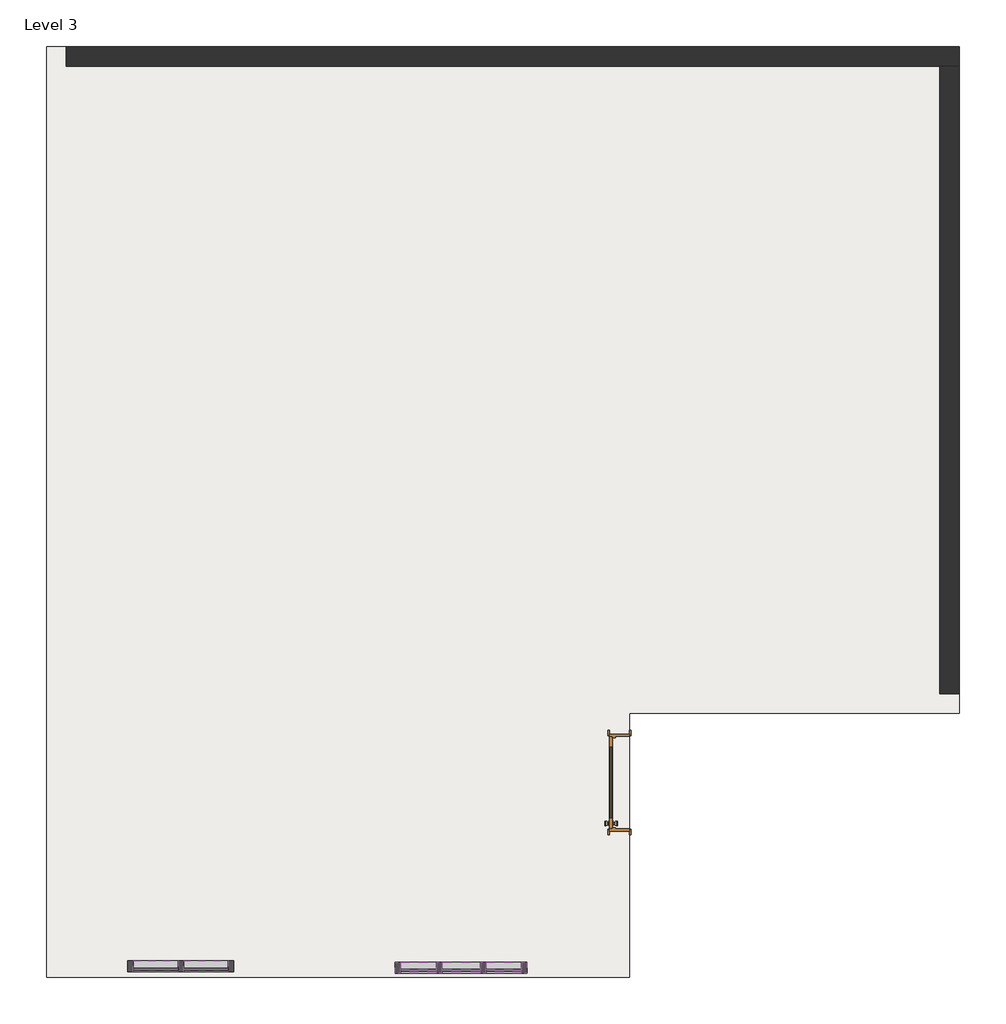
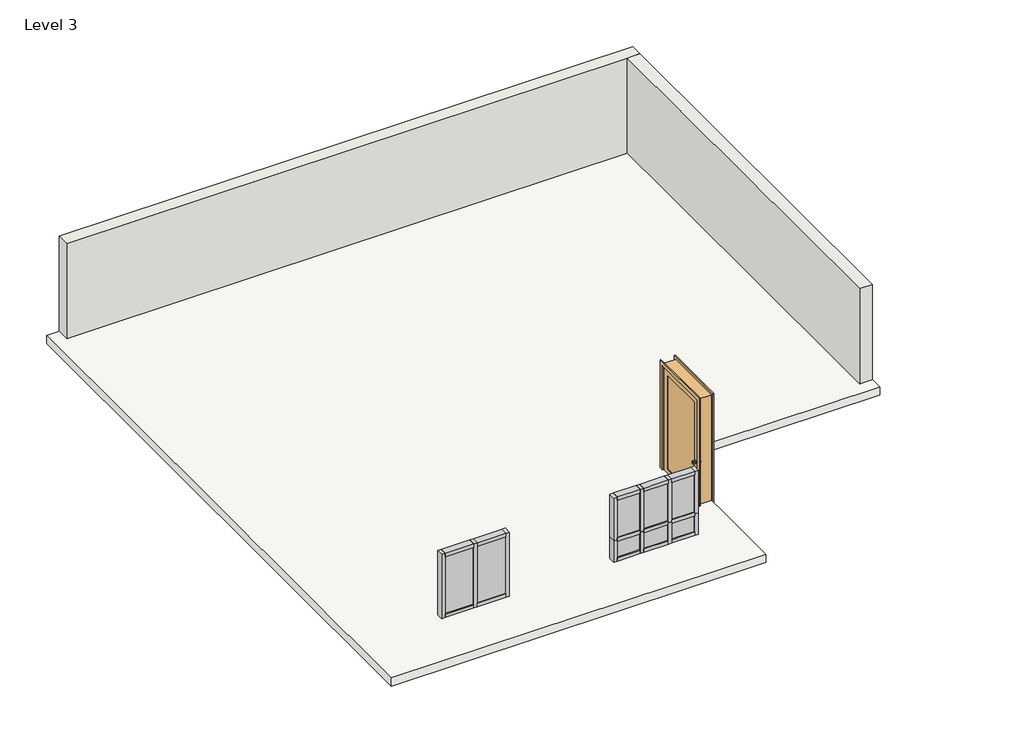
# One storey: 24 members, 8 plates, 2 walls, 1 door, 1 roof.
"""IFC4 building model written with IfcOpenShell, lengths in millimetres."""

from ifc_helpers import new_model, si_unit, frame, origin, place, context, project, spatial, polyline, outline, extrude, faceted_brep, transform, mapped, element, save
from components import door_103cf79b, member_0b7646a3, member_2b49869a, member_75074519, member_dc106669, member_90c805a2, member_5ae8a700, member_718fe5d9, member_bc7dbe04, member_58a4a87b, member_8b3492ed, member_7cfea1b5, system_panel_glazed_1715a493, system_panel_glazed_534e268b, system_panel_glazed_145a7978, system_panel_glazed_a6860354, system_panel_glazed_90648ddd

model = new_model("IFC4")

# Units and contexts
model_context = context("Model", 3, world=origin())
ifc_project = project(units=[si_unit("LENGTHUNIT", "METRE", prefix="MILLI")], contexts=[model_context])

# Site, building, storey
site = spatial("IfcSite", under=ifc_project)
building = spatial("IfcBuilding", under=site)
storey = spatial("IfcBuildingStorey", under=building, Name="Level 3", Elevation=3657.6)

# Door
placement = place(None, origin())
door_shape = door_103cf79b(model_context)
element("IfcDoor", 1, ObjectType="Door-Interior-Single-1_Panel-Wood : 3'6\" x 7'", at=placement, inside=storey, context=model_context, shape_type="MappedRepresentation", body=[
    mapped(door_shape, transform((-5484.7968714, -148.5569638, 3657.6), x_axis=(0.0, 1.0, 0.0), y_axis=(-1.0, 0.0, 0.0), z_axis=(0.0, 0.0, 1.0))),
])

# Members
member_shape = member_0b7646a3(model_context)
element("IfcMember", 2, ObjectType="Rectangular Mullion : 2.5\" x 5\" rectangular", at=placement, inside=storey, context=model_context, shape_type="MappedRepresentation", body=[
    mapped(member_shape, transform((-11095.0218714, -2269.4569638, 5791.2), x_axis=(0.0, 0.0, 1.0), y_axis=(0.0, 1.0, 0.0), z_axis=(-1.0, 0.0, 0.0))),
])
element("IfcMember", 3, ObjectType="Rectangular Mullion : 2.5\" x 5\" rectangular", at=placement, inside=storey, context=model_context, shape_type="MappedRepresentation", body=[
    mapped(member_shape, transform((-10517.1718714, -2269.4569638, 5791.2), x_axis=(0.0, 0.0, 1.0), y_axis=(0.0, 1.0, 0.0), z_axis=(-1.0, 0.0, 0.0))),
])
element("IfcMember", 4, ObjectType="Rectangular Mullion : 2.5\" x 5\" rectangular", at=placement, inside=storey, context=model_context, shape_type="MappedRepresentation", body=[
    mapped(member_shape, transform((-10002.8218714, -2269.4569638, 4572.0), x_axis=(0.0, 0.0, -1.0), y_axis=(0.0, 1.0, 0.0), z_axis=(1.0, 0.0, 0.0))),
])
element("IfcMember", 5, ObjectType="Rectangular Mullion : 2.5\" x 5\" rectangular", at=placement, inside=storey, context=model_context, shape_type="MappedRepresentation", body=[
    mapped(member_shape, transform((-10580.6718714, -2269.4569638, 4572.0), x_axis=(0.0, 0.0, -1.0), y_axis=(0.0, 1.0, 0.0), z_axis=(1.0, 0.0, 0.0))),
])
member_2_shape = member_2b49869a(model_context)
element("IfcMember", 6, ObjectType="Rectangular Mullion : 2.5\" x 5\" rectangular", at=placement, inside=storey, context=model_context, shape_type="MappedRepresentation", body=[
    mapped(member_2_shape, transform((-10548.9218714, -2269.4569638, 4572.0), x_axis=(-1.0, 0.0, 0.0), y_axis=(0.0, 1.0, 0.0), z_axis=(0.0, 0.0, -1.0))),
])
member_3_shape = member_75074519(model_context)
element("IfcMember", 7, ObjectType="Rectangular Mullion : 2.5\" x 5\" rectangular", at=placement, inside=storey, context=model_context, shape_type="MappedRepresentation", body=[
    mapped(member_3_shape, transform((-9939.3218714, -2269.4569638, 5791.2), x_axis=(1.0, 0.0, 0.0), y_axis=(0.0, 1.0, 0.0), z_axis=(0.0, 0.0, 1.0))),
])
element("IfcMember", 8, ObjectType="Rectangular Mullion : 2.5\" x 5\" rectangular", at=placement, inside=storey, context=model_context, shape_type="MappedRepresentation", body=[
    mapped(member_3_shape, transform((-11158.5218714, -2269.4569638, 4572.0), x_axis=(-1.0, 0.0, 0.0), y_axis=(0.0, 1.0, 0.0), z_axis=(0.0, 0.0, -1.0))),
])
member_4_shape = member_dc106669(model_context)
element("IfcMember", 9, ObjectType="Rectangular Mullion : 2.5\" x 5\" rectangular", at=placement, inside=storey, context=model_context, shape_type="MappedRepresentation", body=[
    mapped(member_4_shape, transform((-8008.9218714, -2282.1569638, 5791.2), x_axis=(0.0, 0.0, 1.0), y_axis=(0.0, 1.0, 0.0), z_axis=(-1.0, 0.0, 0.0))),
])
element("IfcMember", 10, ObjectType="Rectangular Mullion : 2.5\" x 5\" rectangular", at=placement, inside=storey, context=model_context, shape_type="MappedRepresentation", body=[
    mapped(member_4_shape, transform((-7024.6718714, -2282.1569638, 5791.2), x_axis=(0.0, 0.0, 1.0), y_axis=(0.0, 1.0, 0.0), z_axis=(-1.0, 0.0, 0.0))),
])
element("IfcMember", 11, ObjectType="Rectangular Mullion : 2.5\" x 5\" rectangular", at=placement, inside=storey, context=model_context, shape_type="MappedRepresentation", body=[
    mapped(member_4_shape, transform((-6611.9218714, -2282.1569638, 4572.0), x_axis=(0.0, 0.0, -1.0), y_axis=(0.0, 1.0, 0.0), z_axis=(1.0, 0.0, 0.0))),
])
element("IfcMember", 12, ObjectType="Rectangular Mullion : 2.5\" x 5\" rectangular", at=placement, inside=storey, context=model_context, shape_type="MappedRepresentation", body=[
    mapped(member_4_shape, transform((-7596.1718714, -2282.1569638, 4572.0), x_axis=(0.0, 0.0, -1.0), y_axis=(0.0, 1.0, 0.0), z_axis=(1.0, 0.0, 0.0))),
])
member_5_shape = member_90c805a2(model_context)
element("IfcMember", 13, ObjectType="Rectangular Mullion : 2.5\" x 5\" rectangular", at=placement, inside=storey, context=model_context, shape_type="MappedRepresentation", body=[
    mapped(member_5_shape, transform((-7564.4218714, -2282.1569638, 4572.0), x_axis=(-1.0, 0.0, 0.0), y_axis=(0.0, 1.0, 0.0), z_axis=(0.0, 0.0, -1.0))),
])
element("IfcMember", 14, ObjectType="Rectangular Mullion : 2.5\" x 5\" rectangular", at=placement, inside=storey, context=model_context, shape_type="MappedRepresentation", body=[
    mapped(member_5_shape, transform((-7056.4218714, -2282.1569638, 4572.0), x_axis=(-1.0, 0.0, 0.0), y_axis=(0.0, 1.0, 0.0), z_axis=(0.0, 0.0, -1.0))),
])
member_6_shape = member_5ae8a700(model_context)
element("IfcMember", 15, ObjectType="Rectangular Mullion : 2.5\" x 5\" rectangular", at=placement, inside=storey, context=model_context, shape_type="MappedRepresentation", body=[
    mapped(member_6_shape, transform((-7024.6718714, -2282.1569638, 4978.4), x_axis=(0.0, 0.0, 1.0), y_axis=(0.0, 1.0, 0.0), z_axis=(-1.0, 0.0, 0.0))),
])
element("IfcMember", 16, ObjectType="Rectangular Mullion : 2.5\" x 5\" rectangular", at=placement, inside=storey, context=model_context, shape_type="MappedRepresentation", body=[
    mapped(member_6_shape, transform((-8008.9218714, -2282.1569638, 4978.4), x_axis=(0.0, 0.0, 1.0), y_axis=(0.0, 1.0, 0.0), z_axis=(-1.0, 0.0, 0.0))),
])
member_7_shape = member_718fe5d9(model_context)
element("IfcMember", 17, ObjectType="Rectangular Mullion : 2.5\" x 5\" rectangular", at=placement, inside=storey, context=model_context, shape_type="MappedRepresentation", body=[
    mapped(member_7_shape, transform((-7532.6718714, -2282.1569638, 4978.4), x_axis=(0.0, 0.0, 1.0), y_axis=(0.0, 1.0, 0.0), z_axis=(-1.0, 0.0, 0.0))),
])
member_8_shape = member_bc7dbe04(model_context)
element("IfcMember", 18, ObjectType="Rectangular Mullion : 2.5\" x 5\" rectangular", at=placement, inside=storey, context=model_context, shape_type="MappedRepresentation", body=[
    mapped(member_8_shape, transform((-7088.1718714, -2282.1569638, 4572.0), x_axis=(0.0, 0.0, -1.0), y_axis=(0.0, 1.0, 0.0), z_axis=(1.0, 0.0, 0.0))),
])
element("IfcMember", 19, ObjectType="Rectangular Mullion : 2.5\" x 5\" rectangular", at=placement, inside=storey, context=model_context, shape_type="MappedRepresentation", body=[
    mapped(member_8_shape, transform((-7532.6718714, -2282.1569638, 5791.2), x_axis=(0.0, 0.0, 1.0), y_axis=(0.0, 1.0, 0.0), z_axis=(-1.0, 0.0, 0.0))),
])
member_9_shape = member_58a4a87b(model_context)
element("IfcMember", 20, ObjectType="Rectangular Mullion : 2.5\" x 5\" rectangular", at=placement, inside=storey, context=model_context, shape_type="MappedRepresentation", body=[
    mapped(member_9_shape, transform((-7564.4218714, -2282.1569638, 4978.4), x_axis=(-1.0, 0.0, 0.0), y_axis=(0.0, 1.0, 0.0), z_axis=(0.0, 0.0, -1.0))),
])
element("IfcMember", 21, ObjectType="Rectangular Mullion : 2.5\" x 5\" rectangular", at=placement, inside=storey, context=model_context, shape_type="MappedRepresentation", body=[
    mapped(member_9_shape, transform((-7056.4218714, -2282.1569638, 4978.4), x_axis=(-1.0, 0.0, 0.0), y_axis=(0.0, 1.0, 0.0), z_axis=(0.0, 0.0, -1.0))),
])
member_10_shape = member_8b3492ed(model_context)
element("IfcMember", 22, ObjectType="Rectangular Mullion : 2.5\" x 5\" rectangular", at=placement, inside=storey, context=model_context, shape_type="MappedRepresentation", body=[
    mapped(member_10_shape, transform((-6548.4218714, -2282.1569638, 5791.2), x_axis=(1.0, 0.0, 0.0), y_axis=(0.0, 1.0, 0.0), z_axis=(0.0, 0.0, 1.0))),
])
member_11_shape = member_7cfea1b5(model_context)
element("IfcMember", 23, ObjectType="Rectangular Mullion : 2.5\" x 5\" rectangular", at=placement, inside=storey, context=model_context, shape_type="MappedRepresentation", body=[
    mapped(member_11_shape, transform((-8072.4218714, -2282.1569638, 4572.0), x_axis=(-1.0, 0.0, 0.0), y_axis=(0.0, 1.0, 0.0), z_axis=(0.0, 0.0, -1.0))),
])
element("IfcMember", 24, ObjectType="Rectangular Mullion : 2.5\" x 5\" rectangular", at=placement, inside=storey, context=model_context, shape_type="MappedRepresentation", body=[
    mapped(member_10_shape, transform((-8072.4218714, -2282.1569638, 4978.4), x_axis=(-1.0, 0.0, 0.0), y_axis=(0.0, 1.0, 0.0), z_axis=(0.0, 0.0, -1.0))),
])
element("IfcMember", 25, ObjectType="Rectangular Mullion : 2.5\" x 5\" rectangular", at=placement, inside=storey, context=model_context, shape_type="MappedRepresentation", body=[
    mapped(member_11_shape, transform((-6548.4218714, -2282.1569638, 4978.4), x_axis=(1.0, 0.0, 0.0), y_axis=(0.0, 1.0, 0.0), z_axis=(0.0, 0.0, 1.0))),
])

# Plates
system_panel_glazed_shape = system_panel_glazed_1715a493(model_context)
element("IfcPlate", 26, ObjectType="System Panel : Glazed", at=placement, inside=storey, context=model_context, shape_type="MappedRepresentation", body=[
    mapped(system_panel_glazed_shape, transform((-10259.9968714, -2269.4569638, 4635.5), x_axis=(-1.0, 0.0, 0.0), y_axis=(0.0, -1.0, 0.0), z_axis=(0.0, 0.0, 1.0))),
])
element("IfcPlate", 27, ObjectType="System Panel : Glazed", at=placement, inside=storey, context=model_context, shape_type="MappedRepresentation", body=[
    mapped(system_panel_glazed_shape, transform((-10837.8468714, -2269.4569638, 4635.5), x_axis=(-1.0, 0.0, 0.0), y_axis=(0.0, -1.0, 0.0), z_axis=(0.0, 0.0, 1.0))),
])
system_panel_glazed_2_shape = system_panel_glazed_534e268b(model_context)
element("IfcPlate", 28, ObjectType="System Panel : Glazed", at=placement, inside=storey, context=model_context, shape_type="MappedRepresentation", body=[
    mapped(system_panel_glazed_2_shape, transform((-6818.2968714, -2282.1569638, 4635.5), x_axis=(-1.0, 0.0, 0.0), y_axis=(0.0, -1.0, 0.0), z_axis=(0.0, 0.0, 1.0))),
])
element("IfcPlate", 29, ObjectType="System Panel : Glazed", at=placement, inside=storey, context=model_context, shape_type="MappedRepresentation", body=[
    mapped(system_panel_glazed_2_shape, transform((-7802.5468714, -2282.1569638, 4635.5), x_axis=(-1.0, 0.0, 0.0), y_axis=(0.0, -1.0, 0.0), z_axis=(0.0, 0.0, 1.0))),
])
system_panel_glazed_3_shape = system_panel_glazed_145a7978(model_context)
element("IfcPlate", 30, ObjectType="System Panel : Glazed", at=placement, inside=storey, context=model_context, shape_type="MappedRepresentation", body=[
    mapped(system_panel_glazed_3_shape, transform((-7310.4218714, -2282.1569638, 4635.5), x_axis=(-1.0, 0.0, 0.0), y_axis=(0.0, -1.0, 0.0), z_axis=(0.0, 0.0, 1.0))),
])
system_panel_glazed_4_shape = system_panel_glazed_a6860354(model_context)
element("IfcPlate", 31, ObjectType="System Panel : Glazed", at=placement, inside=storey, context=model_context, shape_type="MappedRepresentation", body=[
    mapped(system_panel_glazed_4_shape, transform((-6818.2968714, -2282.1569638, 5010.15), x_axis=(-1.0, 0.0, 0.0), y_axis=(0.0, -1.0, 0.0), z_axis=(0.0, 0.0, 1.0))),
])
element("IfcPlate", 32, ObjectType="System Panel : Glazed", at=placement, inside=storey, context=model_context, shape_type="MappedRepresentation", body=[
    mapped(system_panel_glazed_4_shape, transform((-7802.5468714, -2282.1569638, 5010.15), x_axis=(-1.0, 0.0, 0.0), y_axis=(0.0, -1.0, 0.0), z_axis=(0.0, 0.0, 1.0))),
])
system_panel_glazed_5_shape = system_panel_glazed_90648ddd(model_context)
element("IfcPlate", 33, ObjectType="System Panel : Glazed", at=placement, inside=storey, context=model_context, shape_type="MappedRepresentation", body=[
    mapped(system_panel_glazed_5_shape, transform((-7310.4218714, -2282.1569638, 5010.15), x_axis=(-1.0, 0.0, 0.0), y_axis=(0.0, -1.0, 0.0), z_axis=(0.0, 0.0, 1.0))),
])

# Roof
element("IfcRoof", 34, ObjectType="6\"", at=placement, inside=storey, context=model_context, shape_type="SweptSolid", body=[
    extrude(outline(polyline([(-12098.3218714, 8347.7430362), (-1557.3218714, 8347.7430362), (-1557.3218714, 651.5430362), (-5367.3218714, 651.5430362), (-5367.3218714, -2396.4569638), (-12098.3218714, -2396.4569638), (-12098.3218714, 8347.7430362)])), frame((0.0, 0.0, 3657.6), z_axis=(0.0, 0.0, 1.0), x_axis=(1.0, 0.0, 0.0)), (0.0, 0.0, 1.0), 152.4),
])

# Walls
element("IfcWall", 35, ObjectType="9\" wall", at=placement, inside=storey, context=model_context, shape_type="Brep", body=[
    faceted_brep([(-11869.7218714, 8119.1430362, 3657.6), (-1785.9218714, 8119.1430362, 3657.6), (-1557.3218714, 8119.1430362, 3657.6), (-1557.3218714, 8119.1430362, 5621.6075521), (-1785.9218714, 8119.1430362, 5621.6075521), (-11869.7218714, 8119.1430362, 5621.6075521), (-11869.7218714, 8347.7430362, 3657.6), (-11869.7218714, 8347.7430362, 5621.6075521), (-1557.3218714, 8347.7430362, 5621.6075521), (-1557.3218714, 8347.7430362, 3657.6), (-1785.9218714, 8347.7430362, 3657.6)], [[[0, 1, 2, 3, 4, 5]], [[6, 7, 8, 9, 10]], [[2, 1, 0, 6, 10, 9]], [[5, 4, 3, 8, 7]], [[0, 5, 7, 6]], [[3, 2, 9, 8]]]),
])
element("IfcWall", 36, ObjectType="9\" wall", at=placement, inside=storey, context=model_context, shape_type="SweptSolid", body=[
    extrude(outline(polyline([(-1785.9218714, 880.1430362), (-1785.9218714, 8119.1430362), (-1557.3218714, 8119.1430362), (-1557.3218714, 880.1430362), (-1785.9218714, 880.1430362)])), frame((0.0, 0.0, 3657.6), z_axis=(0.0, 0.0, 1.0), x_axis=(1.0, 0.0, 0.0)), (0.0, 0.0, 1.0), 1964.0075521),
])

save(model, "model.ifc")

# Revit data of these elements
# Type "Door-Interior-Single-1_Panel-Wood : 3'6\" x 7'"
#   Type Mark = "9"
#   Assembly Code = "C1020300"
#   Analytic Construction = "Wooden"
#   Top Rail = 0' - 4 11/16"
#   Thickness = 0' - 1 3/8"
#   Thermal Resistance (R) = 2.5876 (h·ft²·°F)/BTU
#   Swing Angle [instance default] = 90.00°
#   Stiles = 0' - 4 3/4"
#   Rough Width = 3' - 8"
#   Rough Height = 7' - 1"
#   Height = 7' - 0"
#   Width = 3' - 6"
#   Heat Transfer Coefficient (U) = 0.3865 BTU/(h·ft²·°F)
#   Bottom Rail = 0' - 9 1/8"
#   Trim Material = Cherry
#   Panel Material = Cherry
#   Frame Material = Cherry
#   Door Handle Material = Aluminum
#   Visual Light Transmittance = 0
#   Solar Heat Gain Coefficient = 0
#   Wall Closure = (empty or 0)
#   Function = (empty or 0)
# Type "Rectangular Mullion : 2.5\" x 5\" rectangular"
#   built-in parameter 1007304 = 0.416667 (stored number, unit not read)
#   built-in parameter 1007301 = 0.104167 (stored number, unit not read)
#   built-in parameter 1007300 = 0.104167 (stored number, unit not read)
# Type "System Panel : Glazed"
#   Construction Type Id = "GSP4R"
#   Analytic Construction = "1/8 in Pilkington single glazing"
#   Visual Light Transmittance = 0.9
#   Solar Heat Gain Coefficient = 0.86
#   Heat Transfer Coefficient (U) = 1.18115 BTU/(h·ft²·°F)
#   Define Thermal Properties by = 1
# Type "6\""
#   Assembly Code = "B1020"
#   Layers, outside or top first: 0' - 6" no material (function 1)
# Type "9\" wall"
#   Assembly Code = "B2010"
#   Layers, outside or top first: 0' - 9" "ash" (function 1)
# Element 1 (IfcDoor, "Door-Interior-Single-1_Panel-Wood : 3'6\" x 7'")
#   Swing Angle = 90.00°
#   Phase Created = New Construction
#   Materials on its faces: "Cherry", "Aluminum"
# Elements 2, 3, 4, 5, 6, 7, 8, 9, 10, 11, 12, 13, 14, 15, 16, 17, 18, 19, 20, 21, 22, 23, 24, 25 (IfcMember, "Rectangular Mullion : 2.5\" x 5\" rectangular")
#   Phase Created = New Construction
# Elements 26, 27, 28, 29, 30, 31, 32, 33 (IfcPlate, "System Panel : Glazed")
#   Phase Created = New Construction
#   Materials on its faces: "Glass"
# Element 34 (IfcRoof, "6\"")
#   built-in parameter 1001705 = 12.5 (stored number, unit not read)
#   built-in parameter 1001710 = 33615
#   Phase Created = New Construction
#   Materials on its faces: "Default Roof"
# Elements 35, 36 (IfcWall, "9\" wall")
#   Top Offset = 5' - 11.32313"
#   Base Offset = 0' - 0"
#   wall height = 6' - 5.32313"
#   Phase Created = New Construction
#   Base Constraint = Level 3
#   Top Constraint = Level 4
#   Materials on its faces: "ash"
# Materials
#   "Cherry": class "Wood", colour RGB 226 177 128, transparency 0, Description = "Prunus Serotina", Cost = 0
#   "Aluminum": class "Metal", colour RGB 247 247 247, transparency 0, Description = "Aluminum 6061", Cost = 0
#   "ash": class "Generic", colour RGB 120 120 120, transparency 0, Cost = 0
#   "Glass": class "Glass", colour RGB 0 128 192, transparency 0.75, Description = "Soda Lime Glass", Cost = 0
#   "Default Roof": colour RGB 88 101 114, transparency 0, Cost = 0
